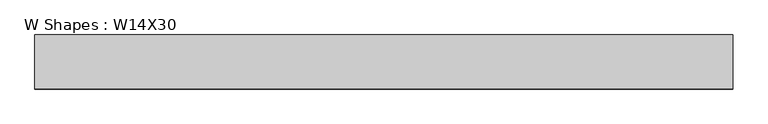
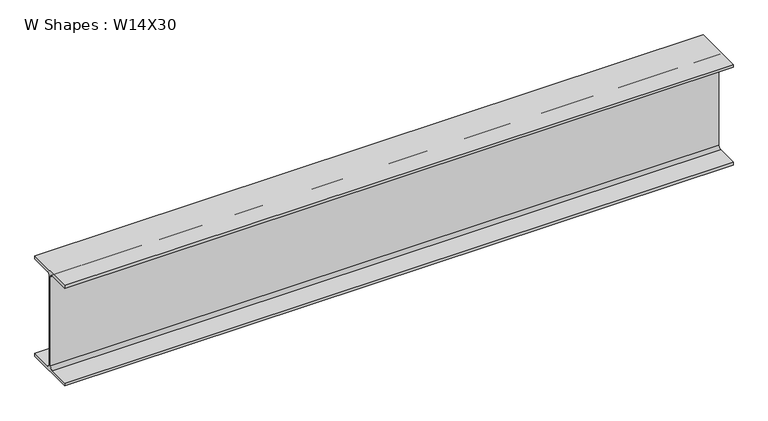
"""IFC4 building model written with IfcOpenShell, lengths in millimetres: beam geometry, W Shapes : W14X30."""

from ifc_helpers import new_model, si_unit, point, frame, frame_2d, origin, place, context, project, spatial, polyline, circle_curve, trimmed, segment, composite_curve, outline, extrude, source, transform, mapped, element, save


def w_shapes_w14x30_23e28ad8(model_context):
    return source(origin(), model_context, "Body", "SweptSolid", [
        extrude(outline(composite_curve([segment(polyline([(85.471, -165.481), (85.471, -175.26), (-85.471, -175.26), (-85.471, -165.481), (-13.589, -165.481)]), True, "CONTINUOUS"), segment(trimmed(circle_curve(frame_2d((-13.589, -155.321)), 10.16), [point((-13.589, -165.481))], [point((-3.429, -155.321))], True, "CARTESIAN"), True, "CONTINUOUS"), segment(polyline([(-3.429, -155.321), (-3.429, 155.321)]), True, "CONTINUOUS"), segment(trimmed(circle_curve(frame_2d((-13.589, 155.321)), 10.16), [point((-3.429, 155.321))], [point((-13.589, 165.481))], True, "CARTESIAN"), True, "CONTINUOUS"), segment(polyline([(-13.589, 165.481), (-85.471, 165.481), (-85.471, 175.26), (85.471, 175.26), (85.471, 165.481), (13.589, 165.481)]), True, "CONTINUOUS"), segment(trimmed(circle_curve(frame_2d((13.589, 155.321)), 10.16), [point((13.589, 165.481))], [point((3.429, 155.321))], True, "CARTESIAN"), True, "CONTINUOUS"), segment(polyline([(3.429, 155.321), (3.429, -155.321)]), True, "CONTINUOUS"), segment(trimmed(circle_curve(frame_2d((13.589, -155.321)), 10.16), [point((3.429, -155.321))], [point((13.589, -165.481))], True, "CARTESIAN"), True, "CONTINUOUS"), segment(polyline([(13.589, -165.481), (85.471, -165.481)]), True, "CONTINUOUS")], self_intersect=False)), frame((-966.4964748, 0.0, 0.0), z_axis=(1.0, 0.0, 0.0), x_axis=(0.0, 1.0, 0.0)), (0.0, 0.0, 1.0), 2206.7425597),
    ])


if __name__ == "__main__":
    model = new_model("IFC4")
    model_context = context("Model", 3, world=origin())
    ifc_project = project(units=[si_unit("LENGTHUNIT", "METRE", prefix="MILLI")], contexts=[model_context])
    site = spatial("IfcSite", under=ifc_project)
    building = spatial("IfcBuilding", under=site)
    placement = place(None, origin())
    w_shapes_w14x30_shape = w_shapes_w14x30_23e28ad8(model_context)
    element("IfcBeam", 1, ObjectType="W Shapes : W14X30", at=placement, inside=building, context=model_context, shape_type="MappedRepresentation", body=[
        mapped(w_shapes_w14x30_shape, transform((0.0, 0.0, 0.0), x_axis=(1.0, 0.0, 0.0), y_axis=(0.0, 1.0, 0.0), z_axis=(0.0, 0.0, 1.0))),
    ])
    save(model, "model.ifc")

# Revit data of these elements
# Type "W Shapes : W14X30"
#   Section Name Key = "W14X30"
#   Width = 6.730"
#   Web Thickness = 0.270"
#   Web Fillet = 0.400"
#   Warping Constant = 887.00 in⁶
#   Torsional Moment of Inertia = 0.38 in⁴
#   Section Area = 8.85 in²
#   Plastic Modulus weak axis = 8.99 in³
#   Plastic Modulus strong axis = 47.30 in³
#   Perimeter = 4.441 ft²/ft
#   Nominal Weight = 30.00 lbf/ft
#   Moment of Inertia weak axis = 19.60 in⁴
#   Moment of Inertia strong axis = 291.00 in⁴
#   Height = 13.800"
#   Flange Thickness = 0.385"
#   Elastic Modulus weak axis = 5.82 in³
#   Elastic Modulus strong axis = 42.00 in³
#   Clear Web Height = 0' - 11 5/8"
#   Centroid Vertical = 6.900"
#   Centroid Horizontal = 3.365"
#   Bolt Spacing = 0' - 3 1/2"
#   Length [instance default] = 1524 mm
#   Structural Material [instance default] = Steel ASTM A992
#   Principal Axes Angle = 0
# Element 1 (IfcBeam, "W Shapes : W14X30")
#   Length = 3476.809 mm
#   Materials on its faces: "Steel ASTM A992"
# Materials
#   "Steel ASTM A992": class "Metal", colour RGB 199 199 199, transparency 0, Description = "Structural steel 50ksi", Cost = 0
